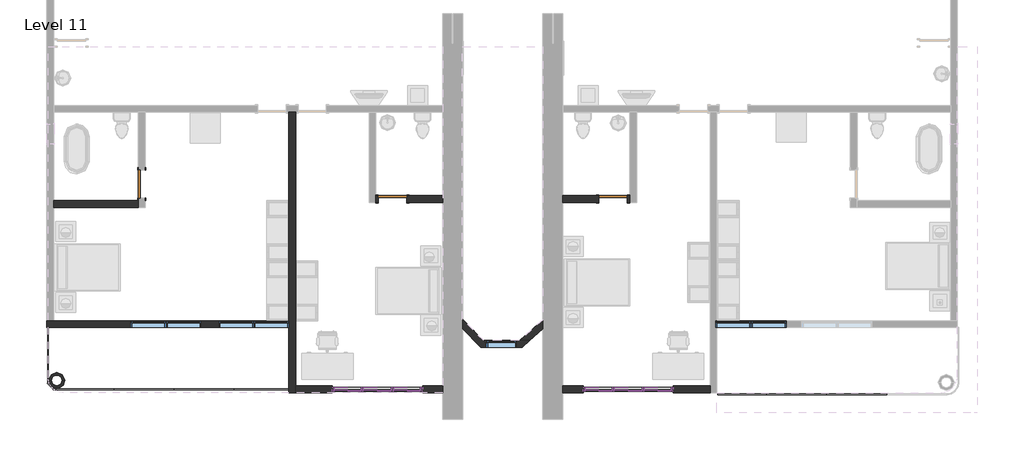
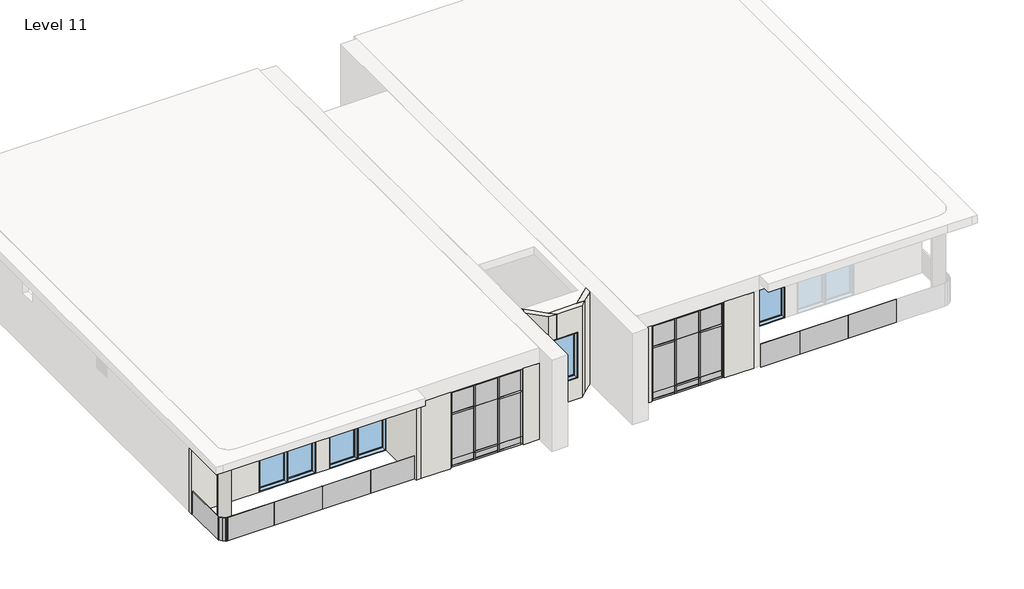
# One storey, part 1 of 3: 42 members, 30 plates, 14 walls, 7 windows, 3 doors.
"""IFC4 building model written with IfcOpenShell, lengths in millimetres."""

from ifc_helpers import new_model, si_unit, point, frame, frame_2d, origin, place, context, project, spatial, polyline, circle_curve, trimmed, segment, composite_curve, outline, extrude, faceted_brep, transform, mapped, element, save
from components import door_2703ae13, door_10fd3a06, member_c17f1be2, member_ad567e07, member_d2e7e466, member_7db1855a, member_75d1e245, member_d60e8053, member_3c3dc66a, member_2fae0574, member_410c6227, member_73c23c35, system_panel_glazed_38d54ecf, system_panel_glazed_fbb6c980, system_panel_glazed_4137532c, system_panel_glazed_6230de04, system_panel_glazed_a79f7f85, system_panel_glazed_9a5ea490, system_panel_glazed_95be5de7, system_panel_glazed_1e00a1c5, system_panel_glazed_ffe51582, system_panel_glazed_8f95e3f6, system_panel_glazed_836907cd, system_panel_glazed_688a65a2, system_panel_glazed_c1a1c740, system_panel_glazed_22bcd51f, window_9a779fa2, window_1a213a25

model = new_model("IFC4")

# Units and contexts
model_context = context("Model", 3, world=origin())
ifc_project = project(units=[si_unit("LENGTHUNIT", "METRE", prefix="MILLI")], contexts=[model_context])

# Site, building, storey
site = spatial("IfcSite", under=ifc_project)
building = spatial("IfcBuilding", under=site)
storey = spatial("IfcBuildingStorey", under=building, Name="Level 11", Elevation=36576.0)

# Doors
placement = place(None, origin())
door_shape = door_2703ae13(model_context)
element("IfcDoor", 1, ObjectType="Door-Single-Panel.0001 : 34\" x 80\"", at=placement, inside=storey, context=model_context, shape_type="MappedRepresentation", body=[
    mapped(door_shape, transform((-15759.6487704, -441.9241442, 36576.0), x_axis=(0.0, -1.0, 0.0), y_axis=(1.0, 0.0, 0.0), z_axis=(0.0, 0.0, 1.0))),
])
element("IfcDoor", 2, ObjectType="Door-Single-Panel.0001 : 34\" x 80\"", at=placement, inside=storey, context=model_context, shape_type="MappedRepresentation", body=[
    mapped(door_shape, transform((-8139.6487704, -899.1241442, 36576.0), x_axis=(-1.0, 0.0, 0.0), y_axis=(0.0, -1.0, 0.0), z_axis=(0.0, 0.0, 1.0))),
])
door_2_shape = door_10fd3a06(model_context)
element("IfcDoor", 3, ObjectType="Door-Single-Panel.0001 : 34\" x 80\"", at=placement, inside=storey, context=model_context, shape_type="MappedRepresentation", body=[
    mapped(door_2_shape, transform((-1434.0487704, -899.1241442, 36576.0), x_axis=(1.0, 0.0, 0.0), y_axis=(0.0, 1.0, 0.0), z_axis=(0.0, 0.0, 1.0))),
])

# Members
member_shape = member_c17f1be2(model_context)
element("IfcMember", 4, ObjectType="Rectangular Mullion : 2.5\" x 5\" rectangular", at=placement, inside=storey, context=model_context, shape_type="MappedRepresentation", body=[
    mapped(member_shape, transform((-9904.9487704, -6690.3241442, 39624.0), x_axis=(0.0, 0.0, 1.0), y_axis=(0.0, 1.0, 0.0), z_axis=(-1.0, 0.0, 0.0))),
])
element("IfcMember", 5, ObjectType="Rectangular Mullion : 2.5\" x 5\" rectangular", at=placement, inside=storey, context=model_context, shape_type="MappedRepresentation", body=[
    mapped(member_shape, transform((-8107.8987704, -6690.3241442, 39624.0), x_axis=(0.0, 0.0, 1.0), y_axis=(0.0, 1.0, 0.0), z_axis=(-1.0, 0.0, 0.0))),
])
element("IfcMember", 6, ObjectType="Rectangular Mullion : 2.5\" x 5\" rectangular", at=placement, inside=storey, context=model_context, shape_type="MappedRepresentation", body=[
    mapped(member_shape, transform((-2284.9487704, -6690.3241442, 39624.0), x_axis=(0.0, 0.0, 1.0), y_axis=(0.0, 1.0, 0.0), z_axis=(-1.0, 0.0, 0.0))),
])
element("IfcMember", 7, ObjectType="Rectangular Mullion : 2.5\" x 5\" rectangular", at=placement, inside=storey, context=model_context, shape_type="MappedRepresentation", body=[
    mapped(member_shape, transform((-487.8987704, -6690.3241442, 39624.0), x_axis=(0.0, 0.0, 1.0), y_axis=(0.0, 1.0, 0.0), z_axis=(-1.0, 0.0, 0.0))),
])
element("IfcMember", 8, ObjectType="Rectangular Mullion : 2.5\" x 5\" rectangular", at=placement, inside=storey, context=model_context, shape_type="MappedRepresentation", body=[
    mapped(member_shape, transform((-7288.7487704, -6690.3241442, 36576.0), x_axis=(0.0, 0.0, -1.0), y_axis=(0.0, 1.0, 0.0), z_axis=(1.0, 0.0, 0.0))),
])
element("IfcMember", 9, ObjectType="Rectangular Mullion : 2.5\" x 5\" rectangular", at=placement, inside=storey, context=model_context, shape_type="MappedRepresentation", body=[
    mapped(member_shape, transform((-9085.7987704, -6690.3241442, 36576.0), x_axis=(0.0, 0.0, -1.0), y_axis=(0.0, 1.0, 0.0), z_axis=(1.0, 0.0, 0.0))),
])
element("IfcMember", 10, ObjectType="Rectangular Mullion : 2.5\" x 5\" rectangular", at=placement, inside=storey, context=model_context, shape_type="MappedRepresentation", body=[
    mapped(member_shape, transform((331.2512296, -6690.3241442, 36576.0), x_axis=(0.0, 0.0, -1.0), y_axis=(0.0, 1.0, 0.0), z_axis=(1.0, 0.0, 0.0))),
])
element("IfcMember", 11, ObjectType="Rectangular Mullion : 2.5\" x 5\" rectangular", at=placement, inside=storey, context=model_context, shape_type="MappedRepresentation", body=[
    mapped(member_shape, transform((-1465.7987704, -6690.3241442, 36576.0), x_axis=(0.0, 0.0, -1.0), y_axis=(0.0, 1.0, 0.0), z_axis=(1.0, 0.0, 0.0))),
])
member_2_shape = member_ad567e07(model_context)
element("IfcMember", 12, ObjectType="Rectangular Mullion : 2.5\" x 5\" rectangular", at=placement, inside=storey, context=model_context, shape_type="MappedRepresentation", body=[
    mapped(member_2_shape, transform((-8107.8987704, -6690.3241442, 38709.6), x_axis=(0.0, 0.0, 1.0), y_axis=(0.0, 1.0, 0.0), z_axis=(-1.0, 0.0, 0.0))),
])
element("IfcMember", 13, ObjectType="Rectangular Mullion : 2.5\" x 5\" rectangular", at=placement, inside=storey, context=model_context, shape_type="MappedRepresentation", body=[
    mapped(member_2_shape, transform((-9904.9487704, -6690.3241442, 38709.6), x_axis=(0.0, 0.0, 1.0), y_axis=(0.0, 1.0, 0.0), z_axis=(-1.0, 0.0, 0.0))),
])
element("IfcMember", 14, ObjectType="Rectangular Mullion : 2.5\" x 5\" rectangular", at=placement, inside=storey, context=model_context, shape_type="MappedRepresentation", body=[
    mapped(member_2_shape, transform((-487.8987704, -6690.3241442, 38709.6), x_axis=(0.0, 0.0, 1.0), y_axis=(0.0, 1.0, 0.0), z_axis=(-1.0, 0.0, 0.0))),
])
element("IfcMember", 15, ObjectType="Rectangular Mullion : 2.5\" x 5\" rectangular", at=placement, inside=storey, context=model_context, shape_type="MappedRepresentation", body=[
    mapped(member_2_shape, transform((-2284.9487704, -6690.3241442, 38709.6), x_axis=(0.0, 0.0, 1.0), y_axis=(0.0, 1.0, 0.0), z_axis=(-1.0, 0.0, 0.0))),
])
member_3_shape = member_d2e7e466(model_context)
element("IfcMember", 16, ObjectType="Rectangular Mullion : 2.5\" x 5\" rectangular", at=placement, inside=storey, context=model_context, shape_type="MappedRepresentation", body=[
    mapped(member_3_shape, transform((-8171.3987704, -6690.3241442, 36576.0), x_axis=(0.0, 0.0, -1.0), y_axis=(0.0, 1.0, 0.0), z_axis=(1.0, 0.0, 0.0))),
])
element("IfcMember", 17, ObjectType="Rectangular Mullion : 2.5\" x 5\" rectangular", at=placement, inside=storey, context=model_context, shape_type="MappedRepresentation", body=[
    mapped(member_3_shape, transform((-551.3987704, -6690.3241442, 36576.0), x_axis=(0.0, 0.0, -1.0), y_axis=(0.0, 1.0, 0.0), z_axis=(1.0, 0.0, 0.0))),
])
member_4_shape = member_7db1855a(model_context)
element("IfcMember", 18, ObjectType="Rectangular Mullion : 2.5\" x 5\" rectangular", at=placement, inside=storey, context=model_context, shape_type="MappedRepresentation", body=[
    mapped(member_4_shape, transform((-9022.2987704, -6690.3241442, 36880.8), x_axis=(0.0, 0.0, 1.0), y_axis=(0.0, 1.0, 0.0), z_axis=(-1.0, 0.0, 0.0))),
])
element("IfcMember", 19, ObjectType="Rectangular Mullion : 2.5\" x 5\" rectangular", at=placement, inside=storey, context=model_context, shape_type="MappedRepresentation", body=[
    mapped(member_4_shape, transform((-1402.2987704, -6690.3241442, 36880.8), x_axis=(0.0, 0.0, 1.0), y_axis=(0.0, 1.0, 0.0), z_axis=(-1.0, 0.0, 0.0))),
])
element("IfcMember", 20, ObjectType="Rectangular Mullion : 2.5\" x 5\" rectangular", at=placement, inside=storey, context=model_context, shape_type="MappedRepresentation", body=[
    mapped(member_3_shape, transform((-9022.2987704, -6690.3241442, 39624.0), x_axis=(0.0, 0.0, 1.0), y_axis=(0.0, 1.0, 0.0), z_axis=(-1.0, 0.0, 0.0))),
])
element("IfcMember", 21, ObjectType="Rectangular Mullion : 2.5\" x 5\" rectangular", at=placement, inside=storey, context=model_context, shape_type="MappedRepresentation", body=[
    mapped(member_3_shape, transform((-1402.2987704, -6690.3241442, 39624.0), x_axis=(0.0, 0.0, 1.0), y_axis=(0.0, 1.0, 0.0), z_axis=(-1.0, 0.0, 0.0))),
])
member_5_shape = member_75d1e245(model_context)
element("IfcMember", 22, ObjectType="Rectangular Mullion : 2.5\" x 5\" rectangular", at=placement, inside=storey, context=model_context, shape_type="MappedRepresentation", body=[
    mapped(member_5_shape, transform((-8139.6487704, -6690.3241442, 36576.0), x_axis=(-1.0, 0.0, 0.0), y_axis=(0.0, 1.0, 0.0), z_axis=(0.0, 0.0, -1.0))),
])
element("IfcMember", 23, ObjectType="Rectangular Mullion : 2.5\" x 5\" rectangular", at=placement, inside=storey, context=model_context, shape_type="MappedRepresentation", body=[
    mapped(member_5_shape, transform((-9054.0487704, -6690.3241442, 36576.0), x_axis=(-1.0, 0.0, 0.0), y_axis=(0.0, 1.0, 0.0), z_axis=(0.0, 0.0, -1.0))),
])
element("IfcMember", 24, ObjectType="Rectangular Mullion : 2.5\" x 5\" rectangular", at=placement, inside=storey, context=model_context, shape_type="MappedRepresentation", body=[
    mapped(member_5_shape, transform((-519.6487704, -6690.3241442, 36576.0), x_axis=(-1.0, 0.0, 0.0), y_axis=(0.0, 1.0, 0.0), z_axis=(0.0, 0.0, -1.0))),
])
element("IfcMember", 25, ObjectType="Rectangular Mullion : 2.5\" x 5\" rectangular", at=placement, inside=storey, context=model_context, shape_type="MappedRepresentation", body=[
    mapped(member_5_shape, transform((-1434.0487704, -6690.3241442, 36576.0), x_axis=(-1.0, 0.0, 0.0), y_axis=(0.0, 1.0, 0.0), z_axis=(0.0, 0.0, -1.0))),
])
member_6_shape = member_d60e8053(model_context)
element("IfcMember", 26, ObjectType="Rectangular Mullion : 2.5\" x 5\" rectangular", at=placement, inside=storey, context=model_context, shape_type="MappedRepresentation", body=[
    mapped(member_6_shape, transform((-8139.6487704, -6690.3241442, 36880.8), x_axis=(-1.0, 0.0, 0.0), y_axis=(0.0, 1.0, 0.0), z_axis=(0.0, 0.0, -1.0))),
])
element("IfcMember", 27, ObjectType="Rectangular Mullion : 2.5\" x 5\" rectangular", at=placement, inside=storey, context=model_context, shape_type="MappedRepresentation", body=[
    mapped(member_6_shape, transform((-9054.0487704, -6690.3241442, 36880.8), x_axis=(-1.0, 0.0, 0.0), y_axis=(0.0, 1.0, 0.0), z_axis=(0.0, 0.0, -1.0))),
])
element("IfcMember", 28, ObjectType="Rectangular Mullion : 2.5\" x 5\" rectangular", at=placement, inside=storey, context=model_context, shape_type="MappedRepresentation", body=[
    mapped(member_6_shape, transform((-519.6487704, -6690.3241442, 36880.8), x_axis=(-1.0, 0.0, 0.0), y_axis=(0.0, 1.0, 0.0), z_axis=(0.0, 0.0, -1.0))),
])
element("IfcMember", 29, ObjectType="Rectangular Mullion : 2.5\" x 5\" rectangular", at=placement, inside=storey, context=model_context, shape_type="MappedRepresentation", body=[
    mapped(member_6_shape, transform((-1434.0487704, -6690.3241442, 36880.8), x_axis=(-1.0, 0.0, 0.0), y_axis=(0.0, 1.0, 0.0), z_axis=(0.0, 0.0, -1.0))),
])
member_7_shape = member_3c3dc66a(model_context)
element("IfcMember", 30, ObjectType="Rectangular Mullion : 2.5\" x 5\" rectangular", at=placement, inside=storey, context=model_context, shape_type="MappedRepresentation", body=[
    mapped(member_7_shape, transform((-9968.4487704, -6690.3241442, 36576.0), x_axis=(-1.0, 0.0, 0.0), y_axis=(0.0, 1.0, 0.0), z_axis=(0.0, 0.0, -1.0))),
])
element("IfcMember", 31, ObjectType="Rectangular Mullion : 2.5\" x 5\" rectangular", at=placement, inside=storey, context=model_context, shape_type="MappedRepresentation", body=[
    mapped(member_7_shape, transform((-2348.4487704, -6690.3241442, 36576.0), x_axis=(-1.0, 0.0, 0.0), y_axis=(0.0, 1.0, 0.0), z_axis=(0.0, 0.0, -1.0))),
])
member_8_shape = member_2fae0574(model_context)
element("IfcMember", 32, ObjectType="Rectangular Mullion : 2.5\" x 5\" rectangular", at=placement, inside=storey, context=model_context, shape_type="MappedRepresentation", body=[
    mapped(member_8_shape, transform((-9968.4487704, -6690.3241442, 36880.8), x_axis=(-1.0, 0.0, 0.0), y_axis=(0.0, 1.0, 0.0), z_axis=(0.0, 0.0, -1.0))),
])
element("IfcMember", 33, ObjectType="Rectangular Mullion : 2.5\" x 5\" rectangular", at=placement, inside=storey, context=model_context, shape_type="MappedRepresentation", body=[
    mapped(member_8_shape, transform((-2348.4487704, -6690.3241442, 36880.8), x_axis=(-1.0, 0.0, 0.0), y_axis=(0.0, 1.0, 0.0), z_axis=(0.0, 0.0, -1.0))),
])
element("IfcMember", 34, ObjectType="Rectangular Mullion : 2.5\" x 5\" rectangular", at=placement, inside=storey, context=model_context, shape_type="MappedRepresentation", body=[
    mapped(member_8_shape, transform((-7225.2487704, -6690.3241442, 38709.6), x_axis=(1.0, 0.0, 0.0), y_axis=(0.0, 1.0, 0.0), z_axis=(0.0, 0.0, 1.0))),
])
element("IfcMember", 35, ObjectType="Rectangular Mullion : 2.5\" x 5\" rectangular", at=placement, inside=storey, context=model_context, shape_type="MappedRepresentation", body=[
    mapped(member_8_shape, transform((394.7512296, -6690.3241442, 38709.6), x_axis=(1.0, 0.0, 0.0), y_axis=(0.0, 1.0, 0.0), z_axis=(0.0, 0.0, 1.0))),
])
element("IfcMember", 36, ObjectType="Rectangular Mullion : 2.5\" x 5\" rectangular", at=placement, inside=storey, context=model_context, shape_type="MappedRepresentation", body=[
    mapped(member_7_shape, transform((-7225.2487704, -6690.3241442, 36880.8), x_axis=(1.0, 0.0, 0.0), y_axis=(0.0, 1.0, 0.0), z_axis=(0.0, 0.0, 1.0))),
])
element("IfcMember", 37, ObjectType="Rectangular Mullion : 2.5\" x 5\" rectangular", at=placement, inside=storey, context=model_context, shape_type="MappedRepresentation", body=[
    mapped(member_7_shape, transform((394.7512296, -6690.3241442, 36880.8), x_axis=(1.0, 0.0, 0.0), y_axis=(0.0, 1.0, 0.0), z_axis=(0.0, 0.0, 1.0))),
])
member_9_shape = member_410c6227(model_context)
element("IfcMember", 38, ObjectType="Rectangular Mullion : 2.5\" x 5\" rectangular", at=placement, inside=storey, context=model_context, shape_type="MappedRepresentation", body=[
    mapped(member_9_shape, transform((-8139.6487704, -6690.3241442, 38709.6), x_axis=(-1.0, 0.0, 0.0), y_axis=(0.0, 1.0, 0.0), z_axis=(0.0, 0.0, -1.0))),
])
element("IfcMember", 39, ObjectType="Rectangular Mullion : 2.5\" x 5\" rectangular", at=placement, inside=storey, context=model_context, shape_type="MappedRepresentation", body=[
    mapped(member_9_shape, transform((-9054.0487704, -6690.3241442, 38709.6), x_axis=(-1.0, 0.0, 0.0), y_axis=(0.0, 1.0, 0.0), z_axis=(0.0, 0.0, -1.0))),
])
element("IfcMember", 40, ObjectType="Rectangular Mullion : 2.5\" x 5\" rectangular", at=placement, inside=storey, context=model_context, shape_type="MappedRepresentation", body=[
    mapped(member_9_shape, transform((-519.6487704, -6690.3241442, 38709.6), x_axis=(-1.0, 0.0, 0.0), y_axis=(0.0, 1.0, 0.0), z_axis=(0.0, 0.0, -1.0))),
])
element("IfcMember", 41, ObjectType="Rectangular Mullion : 2.5\" x 5\" rectangular", at=placement, inside=storey, context=model_context, shape_type="MappedRepresentation", body=[
    mapped(member_9_shape, transform((-1434.0487704, -6690.3241442, 38709.6), x_axis=(-1.0, 0.0, 0.0), y_axis=(0.0, 1.0, 0.0), z_axis=(0.0, 0.0, -1.0))),
])
member_10_shape = member_73c23c35(model_context)
element("IfcMember", 42, ObjectType="Rectangular Mullion : 2.5\" x 5\" rectangular", at=placement, inside=storey, context=model_context, shape_type="MappedRepresentation", body=[
    mapped(member_10_shape, transform((-7225.2487704, -6690.3241442, 39624.0), x_axis=(1.0, 0.0, 0.0), y_axis=(0.0, 1.0, 0.0), z_axis=(0.0, 0.0, 1.0))),
])
element("IfcMember", 43, ObjectType="Rectangular Mullion : 2.5\" x 5\" rectangular", at=placement, inside=storey, context=model_context, shape_type="MappedRepresentation", body=[
    mapped(member_10_shape, transform((394.7512296, -6690.3241442, 39624.0), x_axis=(1.0, 0.0, 0.0), y_axis=(0.0, 1.0, 0.0), z_axis=(0.0, 0.0, 1.0))),
])
element("IfcMember", 44, ObjectType="Rectangular Mullion : 2.5\" x 5\" rectangular", at=placement, inside=storey, context=model_context, shape_type="MappedRepresentation", body=[
    mapped(member_10_shape, transform((-9968.4487704, -6690.3241442, 38709.6), x_axis=(-1.0, 0.0, 0.0), y_axis=(0.0, 1.0, 0.0), z_axis=(0.0, 0.0, -1.0))),
])
element("IfcMember", 45, ObjectType="Rectangular Mullion : 2.5\" x 5\" rectangular", at=placement, inside=storey, context=model_context, shape_type="MappedRepresentation", body=[
    mapped(member_10_shape, transform((-2348.4487704, -6690.3241442, 38709.6), x_axis=(-1.0, 0.0, 0.0), y_axis=(0.0, 1.0, 0.0), z_axis=(0.0, 0.0, -1.0))),
])

# Plates
system_panel_glazed_shape = system_panel_glazed_38d54ecf(model_context)
element("IfcPlate", 46, ObjectType="System Panel : Glazed", at=placement, inside=storey, context=model_context, shape_type="MappedRepresentation", body=[
    mapped(system_panel_glazed_shape, transform((-8596.8487704, -6690.3241442, 36912.55), x_axis=(-1.0, 0.0, 0.0), y_axis=(0.0, -1.0, 0.0), z_axis=(0.0, 0.0, 1.0))),
])
element("IfcPlate", 47, ObjectType="System Panel : Glazed", at=placement, inside=storey, context=model_context, shape_type="MappedRepresentation", body=[
    mapped(system_panel_glazed_shape, transform((-976.8487704, -6690.3241442, 36912.55), x_axis=(-1.0, 0.0, 0.0), y_axis=(0.0, -1.0, 0.0), z_axis=(0.0, 0.0, 1.0))),
])
system_panel_glazed_2_shape = system_panel_glazed_fbb6c980(model_context)
element("IfcPlate", 48, ObjectType="System Panel : Glazed", at=placement, inside=storey, context=model_context, shape_type="MappedRepresentation", body=[
    mapped(system_panel_glazed_2_shape, transform((-8596.8487704, -6690.3241442, 36639.5), x_axis=(-1.0, 0.0, 0.0), y_axis=(0.0, -1.0, 0.0), z_axis=(0.0, 0.0, 1.0))),
])
element("IfcPlate", 49, ObjectType="System Panel : Glazed", at=placement, inside=storey, context=model_context, shape_type="MappedRepresentation", body=[
    mapped(system_panel_glazed_2_shape, transform((-976.8487704, -6690.3241442, 36639.5), x_axis=(-1.0, 0.0, 0.0), y_axis=(0.0, -1.0, 0.0), z_axis=(0.0, 0.0, 1.0))),
])
system_panel_glazed_3_shape = system_panel_glazed_4137532c(model_context)
element("IfcPlate", 50, ObjectType="System Panel : Glazed", at=placement, inside=storey, context=model_context, shape_type="MappedRepresentation", body=[
    mapped(system_panel_glazed_3_shape, transform((-7698.3237704, -6690.3241442, 36639.5), x_axis=(-1.0, 0.0, 0.0), y_axis=(0.0, -1.0, 0.0), z_axis=(0.0, 0.0, 1.0))),
])
element("IfcPlate", 51, ObjectType="System Panel : Glazed", at=placement, inside=storey, context=model_context, shape_type="MappedRepresentation", body=[
    mapped(system_panel_glazed_3_shape, transform((-9495.3737704, -6690.3241442, 36639.5), x_axis=(-1.0, 0.0, 0.0), y_axis=(0.0, -1.0, 0.0), z_axis=(0.0, 0.0, 1.0))),
])
element("IfcPlate", 52, ObjectType="System Panel : Glazed", at=placement, inside=storey, context=model_context, shape_type="MappedRepresentation", body=[
    mapped(system_panel_glazed_3_shape, transform((-78.3237704, -6690.3241442, 36639.5), x_axis=(-1.0, 0.0, 0.0), y_axis=(0.0, -1.0, 0.0), z_axis=(0.0, 0.0, 1.0))),
])
element("IfcPlate", 53, ObjectType="System Panel : Glazed", at=placement, inside=storey, context=model_context, shape_type="MappedRepresentation", body=[
    mapped(system_panel_glazed_3_shape, transform((-1875.3737704, -6690.3241442, 36639.5), x_axis=(-1.0, 0.0, 0.0), y_axis=(0.0, -1.0, 0.0), z_axis=(0.0, 0.0, 1.0))),
])
system_panel_glazed_4_shape = system_panel_glazed_6230de04(model_context)
element("IfcPlate", 54, ObjectType="System Panel : Glazed", at=placement, inside=storey, context=model_context, shape_type="MappedRepresentation", body=[
    mapped(system_panel_glazed_4_shape, transform((-7698.3237704, -6690.3241442, 36880.8), x_axis=(-1.0, 0.0, 0.0), y_axis=(0.0, -1.0, 0.0), z_axis=(0.0, 0.0, 1.0))),
])
element("IfcPlate", 55, ObjectType="System Panel : Glazed", at=placement, inside=storey, context=model_context, shape_type="MappedRepresentation", body=[
    mapped(system_panel_glazed_4_shape, transform((-9495.3737704, -6690.3241442, 36880.8), x_axis=(-1.0, 0.0, 0.0), y_axis=(0.0, -1.0, 0.0), z_axis=(0.0, 0.0, 1.0))),
])
element("IfcPlate", 56, ObjectType="System Panel : Glazed", at=placement, inside=storey, context=model_context, shape_type="MappedRepresentation", body=[
    mapped(system_panel_glazed_4_shape, transform((-78.3237704, -6690.3241442, 36880.8), x_axis=(-1.0, 0.0, 0.0), y_axis=(0.0, -1.0, 0.0), z_axis=(0.0, 0.0, 1.0))),
])
element("IfcPlate", 57, ObjectType="System Panel : Glazed", at=placement, inside=storey, context=model_context, shape_type="MappedRepresentation", body=[
    mapped(system_panel_glazed_4_shape, transform((-1875.3737704, -6690.3241442, 36880.8), x_axis=(-1.0, 0.0, 0.0), y_axis=(0.0, -1.0, 0.0), z_axis=(0.0, 0.0, 1.0))),
])
system_panel_glazed_5_shape = system_panel_glazed_a79f7f85(model_context)
element("IfcPlate", 58, ObjectType="System Panel : Glazed", at=placement, inside=storey, context=model_context, shape_type="MappedRepresentation", body=[
    mapped(system_panel_glazed_5_shape, transform((-7698.3237704, -6690.3241442, 38741.35), x_axis=(-1.0, 0.0, 0.0), y_axis=(0.0, -1.0, 0.0), z_axis=(0.0, 0.0, 1.0))),
])
element("IfcPlate", 59, ObjectType="System Panel : Glazed", at=placement, inside=storey, context=model_context, shape_type="MappedRepresentation", body=[
    mapped(system_panel_glazed_5_shape, transform((-9495.3737704, -6690.3241442, 38741.35), x_axis=(-1.0, 0.0, 0.0), y_axis=(0.0, -1.0, 0.0), z_axis=(0.0, 0.0, 1.0))),
])
element("IfcPlate", 60, ObjectType="System Panel : Glazed", at=placement, inside=storey, context=model_context, shape_type="MappedRepresentation", body=[
    mapped(system_panel_glazed_5_shape, transform((-78.3237704, -6690.3241442, 38741.35), x_axis=(-1.0, 0.0, 0.0), y_axis=(0.0, -1.0, 0.0), z_axis=(0.0, 0.0, 1.0))),
])
element("IfcPlate", 61, ObjectType="System Panel : Glazed", at=placement, inside=storey, context=model_context, shape_type="MappedRepresentation", body=[
    mapped(system_panel_glazed_5_shape, transform((-1875.3737704, -6690.3241442, 38741.35), x_axis=(-1.0, 0.0, 0.0), y_axis=(0.0, -1.0, 0.0), z_axis=(0.0, 0.0, 1.0))),
])
system_panel_glazed_6_shape = system_panel_glazed_9a5ea490(model_context)
element("IfcPlate", 62, ObjectType="System Panel : Glazed", at=placement, inside=storey, context=model_context, shape_type="MappedRepresentation", body=[
    mapped(system_panel_glazed_6_shape, transform((-8596.8487704, -6690.3241442, 38709.6), x_axis=(-1.0, 0.0, 0.0), y_axis=(0.0, -1.0, 0.0), z_axis=(0.0, 0.0, 1.0))),
])
element("IfcPlate", 63, ObjectType="System Panel : Glazed", at=placement, inside=storey, context=model_context, shape_type="MappedRepresentation", body=[
    mapped(system_panel_glazed_6_shape, transform((-976.8487704, -6690.3241442, 38709.6), x_axis=(-1.0, 0.0, 0.0), y_axis=(0.0, -1.0, 0.0), z_axis=(0.0, 0.0, 1.0))),
])
system_panel_glazed_7_shape = system_panel_glazed_95be5de7(model_context)
element("IfcPlate", 64, ObjectType="System Panel : Glazed", at=placement, inside=storey, context=model_context, shape_type="MappedRepresentation", body=[
    mapped(system_panel_glazed_7_shape, transform((-15700.8805745, -6723.6923401, 36576.0), x_axis=(1.0, 0.0, 0.0), y_axis=(0.0, 1.0, 0.0), z_axis=(0.0, 0.0, 1.0))),
])
element("IfcPlate", 65, ObjectType="System Panel : Glazed", at=placement, inside=storey, context=model_context, shape_type="MappedRepresentation", body=[
    mapped(system_panel_glazed_7_shape, transform((-13872.0805745, -6723.6923401, 36576.0), x_axis=(1.0, 0.0, 0.0), y_axis=(0.0, 1.0, 0.0), z_axis=(0.0, 0.0, 1.0))),
])
element("IfcPlate", 66, ObjectType="System Panel : Glazed", at=placement, inside=storey, context=model_context, shape_type="MappedRepresentation", body=[
    mapped(system_panel_glazed_7_shape, transform((5964.2620092, -6810.4133646, 36576.0), x_axis=(-1.0, 0.0, 0.0), y_axis=(0.0, -1.0, 0.0), z_axis=(0.0, 0.0, 1.0))),
])
element("IfcPlate", 67, ObjectType="System Panel : Glazed", at=placement, inside=storey, context=model_context, shape_type="MappedRepresentation", body=[
    mapped(system_panel_glazed_7_shape, transform((4135.4620092, -6810.4133646, 36576.0), x_axis=(-1.0, 0.0, 0.0), y_axis=(0.0, -1.0, 0.0), z_axis=(0.0, 0.0, 1.0))),
])
system_panel_glazed_8_shape = system_panel_glazed_1e00a1c5(model_context)
element("IfcPlate", 68, ObjectType="System Panel : Glazed", at=placement, inside=storey, context=model_context, shape_type="MappedRepresentation", body=[
    mapped(system_panel_glazed_8_shape, transform((2484.4620092, -6810.4133646, 36576.0), x_axis=(-1.0, 0.0, 0.0), y_axis=(0.0, -1.0, 0.0), z_axis=(0.0, 0.0, 1.0))),
])
system_panel_glazed_9_shape = system_panel_glazed_ffe51582(model_context)
element("IfcPlate", 69, ObjectType="System Panel : Glazed", at=placement, inside=storey, context=model_context, shape_type="MappedRepresentation", body=[
    mapped(system_panel_glazed_9_shape, transform((-18445.6213429, -6722.1515718, 36576.0), x_axis=(0.7071067811865462, -0.7071067811865488, 0.0), y_axis=(0.7071067811865488, 0.7071067811865462, 0.0), z_axis=(0.0, 0.0, 1.0))),
])
system_panel_glazed_10_shape = system_panel_glazed_8f95e3f6(model_context)
element("IfcPlate", 70, ObjectType="System Panel : Glazed", at=placement, inside=storey, context=model_context, shape_type="MappedRepresentation", body=[
    mapped(system_panel_glazed_10_shape, transform((-18642.5487704, -5667.9741442, 36576.0), x_axis=(0.0, -1.0, 0.0), y_axis=(1.0, 0.0, 0.0), z_axis=(0.0, 0.0, 1.0))),
])
system_panel_glazed_11_shape = system_panel_glazed_836907cd(model_context)
element("IfcPlate", 71, ObjectType="System Panel : Glazed", at=placement, inside=storey, context=model_context, shape_type="MappedRepresentation", body=[
    mapped(system_panel_glazed_11_shape, transform((-18412.3305745, -6723.6923401, 36576.0), x_axis=(1.0, 0.0, 0.0), y_axis=(0.0, 1.0, 0.0), z_axis=(0.0, 0.0, 1.0))),
])
system_panel_glazed_12_shape = system_panel_glazed_688a65a2(model_context)
element("IfcPlate", 72, ObjectType="System Panel : Glazed", at=placement, inside=storey, context=model_context, shape_type="MappedRepresentation", body=[
    mapped(system_panel_glazed_12_shape, transform((-12123.4646725, -6723.6923401, 36576.0), x_axis=(1.0, 0.0, 0.0), y_axis=(0.0, 1.0, 0.0), z_axis=(0.0, 0.0, 1.0))),
])
system_panel_glazed_13_shape = system_panel_glazed_c1a1c740(model_context)
element("IfcPlate", 73, ObjectType="System Panel : Glazed", at=placement, inside=storey, context=model_context, shape_type="MappedRepresentation", body=[
    mapped(system_panel_glazed_13_shape, transform((-17497.9305745, -6723.6923401, 36576.0), x_axis=(1.0, 0.0, 0.0), y_axis=(0.0, 1.0, 0.0), z_axis=(0.0, 0.0, 1.0))),
])
system_panel_glazed_14_shape = system_panel_glazed_22bcd51f(model_context)
element("IfcPlate", 74, ObjectType="System Panel : Glazed", at=placement, inside=storey, context=model_context, shape_type="MappedRepresentation", body=[
    mapped(system_panel_glazed_14_shape, transform((-18593.7021056, -6574.070809, 36576.0), x_axis=(0.7071067811865462, -0.7071067811865488, 0.0), y_axis=(0.7071067811865488, 0.7071067811865462, 0.0), z_axis=(0.0, 0.0, 1.0))),
])
element("IfcPlate", 75, ObjectType="System Panel : Glazed", at=placement, inside=storey, context=model_context, shape_type="MappedRepresentation", body=[
    mapped(system_panel_glazed_14_shape, transform((-18496.0087761, -6671.7641386, 36576.0), x_axis=(0.7071067811865462, -0.7071067811865488, 0.0), y_axis=(0.7071067811865488, 0.7071067811865462, 0.0), z_axis=(0.0, 0.0, 1.0))),
])

# Walls
element("IfcWall", 76, ObjectType="Generic - 3\" green 2", at=placement, inside=storey, context=model_context, shape_type="SweptSolid", body=[
    extrude(outline(composite_curve([segment(polyline([(-18512.3737704, -6418.8616442), (-18588.5737704, -6418.8616442)]), True, "CONTINUOUS"), segment(trimmed(circle_curve(frame_2d((-18347.2737704, -6418.8616442)), 241.3), [point((-18588.5737704, -6418.8616442))], [point((-18105.9737704, -6418.8616442))], False, "CARTESIAN"), True, "CONTINUOUS"), segment(polyline([(-18105.9737704, -6418.8616442), (-18182.1737704, -6418.8616442)]), True, "CONTINUOUS"), segment(trimmed(circle_curve(frame_2d((-18347.2737704, -6418.8616442)), 165.1), [point((-18182.1737704, -6418.8616442))], [point((-18512.3737704, -6418.8616442))], True, "CARTESIAN"), True, "CONTINUOUS")], self_intersect=False)), frame((0.0, 0.0, 36576.0), z_axis=(0.0, 0.0, 1.0), x_axis=(1.0, 0.0, 0.0)), (0.0, 0.0, 1.0), 3048.0),
])
element("IfcWall", 77, ObjectType="Generic - 3\" green 2", at=placement, inside=storey, context=model_context, shape_type="SweptSolid", body=[
    extrude(outline(composite_curve([segment(polyline([(-18182.1737704, -6418.8616442), (-18105.9737704, -6418.8616442)]), True, "CONTINUOUS"), segment(trimmed(circle_curve(frame_2d((-18347.2737704, -6418.8616442)), 241.3), [point((-18105.9737704, -6418.8616442))], [point((-18588.5737704, -6418.8616442))], False, "CARTESIAN"), True, "CONTINUOUS"), segment(polyline([(-18588.5737704, -6418.8616442), (-18512.3737704, -6418.8616442)]), True, "CONTINUOUS"), segment(trimmed(circle_curve(frame_2d((-18347.2737704, -6418.8616442)), 165.1), [point((-18512.3737704, -6418.8616442))], [point((-18182.1737704, -6418.8616442))], True, "CARTESIAN"), True, "CONTINUOUS")], self_intersect=False)), frame((0.0, 0.0, 36576.0), z_axis=(0.0, 0.0, 1.0), x_axis=(1.0, 0.0, 0.0)), (0.0, 0.0, 1.0), 3048.0),
])
element("IfcWall", 78, ObjectType="Generic - 8\" cream", at=placement, inside=storey, context=model_context, shape_type="Brep", body=[
    faceted_brep([(-11289.2487704, 1742.4758558, 36576.0), (-11289.2487704, -6791.9241442, 36576.0), (-11289.2487704, -6791.9241442, 39624.0), (-11289.2487704, -4810.7241442, 39624.0), (-11289.2487704, -4607.5241442, 39624.0), (-11289.2487704, 1742.4758558, 39624.0), (-11086.0487704, 1742.4758558, 36576.0), (-11086.0487704, 1742.4758558, 39624.0), (-11086.0487704, -6588.7241442, 39624.0), (-11086.0487704, -6791.9241442, 39624.0), (-11086.0487704, -6791.9241442, 36576.0), (-11086.0487704, -6588.7241442, 36576.0)], [[[0, 1, 2, 3, 4, 5]], [[6, 7, 8, 9, 10, 11]], [[1, 0, 6, 11, 10]], [[5, 4, 3, 2, 9, 8, 7]], [[0, 5, 7, 6]], [[2, 1, 10, 9]]]),
])
element("IfcWall", 79, ObjectType="Generic - 8\" cream", at=placement, inside=storey, context=model_context, shape_type="SweptSolid", body=[
    extrude(outline(polyline([(-18439.3487704, -949.9241442), (-15861.2487704, -949.9241442), (-15861.2487704, -1153.1241442), (-18439.3487704, -1153.1241442), (-18439.3487704, -949.9241442)])), frame((0.0, 0.0, 36576.0), z_axis=(0.0, 0.0, 1.0), x_axis=(1.0, 0.0, 0.0)), (0.0, 0.0, 1.0), 3048.0),
])
element("IfcWall", 80, ObjectType="Generic - 8\" cream", at=placement, inside=storey, context=model_context, shape_type="SweptSolid", body=[
    extrude(outline(polyline([(39624.0, -6615.6487704), (39624.0, -8647.6487704), (36576.0, -8647.6487704), (36576.0, -8571.4487704), (38608.0, -8571.4487704), (38608.0, -7707.8487704), (36576.0, -7707.8487704), (36576.0, -6615.6487704), (39624.0, -6615.6487704)])), frame((0.0, -1000.7241442, 0.0), z_axis=(0.0, 1.0, 0.0), x_axis=(0.0, 0.0, 1.0)), (0.0, 0.0, 1.0), 203.2),
])
element("IfcWall", 81, ObjectType="Generic - 8\" cream", at=placement, inside=storey, context=model_context, shape_type="Brep", body=[
    faceted_brep([(-18642.5487704, -4607.5241442, 39624.0), (-18439.3487704, -4607.5241442, 39624.0), (-11289.2487704, -4607.5241442, 39624.0), (-11289.2487704, -4607.5241442, 39319.2), (-13422.8487704, -4607.5241442, 39319.2), (-13422.8487704, -4607.5241442, 36576.0), (-13956.2487704, -4607.5241442, 36576.0), (-13956.2487704, -4607.5241442, 39319.2), (-16089.8487704, -4607.5241442, 39319.2), (-16089.8487704, -4607.5241442, 36576.0), (-18439.3487704, -4607.5241442, 36576.0), (-18642.5487704, -4607.5241442, 36576.0), (-11289.2487704, -4810.7241442, 39624.0), (-18642.5487704, -4810.7241442, 39624.0), (-18642.5487704, -4810.7241442, 36576.0), (-16089.8487704, -4810.7241442, 36576.0), (-16089.8487704, -4810.7241442, 39319.2), (-13956.2487704, -4810.7241442, 39319.2), (-13956.2487704, -4810.7241442, 36576.0), (-13422.8487704, -4810.7241442, 36576.0), (-13422.8487704, -4810.7241442, 39319.2), (-11289.2487704, -4810.7241442, 39319.2)], [[[0, 1, 2, 3, 4, 5, 6, 7, 8, 9, 10, 11]], [[12, 13, 14, 15, 16, 17, 18, 19, 20, 21]], [[14, 11, 10, 9, 15]], [[5, 19, 18, 6]], [[2, 1, 0, 13, 12]], [[2, 12, 21, 3]], [[0, 11, 14, 13]], [[3, 21, 20, 4]], [[4, 20, 19, 5]], [[17, 7, 6, 18]], [[7, 17, 16, 8]], [[8, 16, 15, 9]]]),
])
element("IfcWall", 82, ObjectType="Generic - 8\" cream", at=placement, inside=storey, context=model_context, shape_type="SweptSolid", body=[
    extrude(outline(polyline([(39624.0, -926.0487704), (39624.0, -2958.0487704), (36576.0, -2958.0487704), (36576.0, -1865.8487704), (38608.0, -1865.8487704), (38608.0, -1002.2487704), (36576.0, -1002.2487704), (36576.0, -926.0487704), (39624.0, -926.0487704)])), frame((0.0, -1000.7241442, 0.0), z_axis=(0.0, 1.0, 0.0), x_axis=(0.0, 0.0, 1.0)), (0.0, 0.0, 1.0), 203.2),
])
element("IfcWall", 83, ObjectType="Generic - 8\" cream", at=placement, inside=storey, context=model_context, shape_type="SweptSolid", body=[
    extrude(outline(polyline([(394.7512296, -6588.7241442), (1512.3512296, -6588.7241442), (1512.3512296, -6791.9241442), (394.7512296, -6791.9241442), (394.7512296, -6588.7241442)])), frame((0.0, 0.0, 36576.0), z_axis=(0.0, 0.0, 1.0), x_axis=(1.0, 0.0, 0.0)), (0.0, 0.0, 1.0), 3048.0),
])
element("IfcWall", 84, ObjectType="Generic - 8\" cream", at=placement, inside=storey, context=model_context, shape_type="SweptSolid", body=[
    extrude(outline(polyline([(-2348.4487704, -6791.9241442), (-2958.0487704, -6791.9241442), (-2958.0487704, -6588.7241442), (-2348.4487704, -6588.7241442), (-2348.4487704, -6791.9241442)])), frame((0.0, 0.0, 36576.0), z_axis=(0.0, 0.0, 1.0), x_axis=(1.0, 0.0, 0.0)), (0.0, 0.0, 1.0), 3048.0),
])
element("IfcWall", 85, ObjectType="Generic - 8\" cream", at=placement, inside=storey, context=model_context, shape_type="SweptSolid", body=[
    extrude(outline(polyline([(-9968.4487704, -6791.9241442), (-11086.0487704, -6791.9241442), (-11086.0487704, -6588.7241442), (-9968.4487704, -6588.7241442), (-9968.4487704, -6791.9241442)])), frame((0.0, 0.0, 36576.0), z_axis=(0.0, 0.0, 1.0), x_axis=(1.0, 0.0, 0.0)), (0.0, 0.0, 1.0), 3048.0),
])
element("IfcWall", 86, ObjectType="Generic - 8\" cream", at=placement, inside=storey, context=model_context, shape_type="SweptSolid", body=[
    extrude(outline(polyline([(-7225.2487704, -6588.7241442), (-6615.6487704, -6588.7241442), (-6615.6487704, -6791.9241442), (-7225.2487704, -6791.9241442), (-7225.2487704, -6588.7241442)])), frame((0.0, 0.0, 36576.0), z_axis=(0.0, 0.0, 1.0), x_axis=(1.0, 0.0, 0.0)), (0.0, 0.0, 1.0), 3048.0),
])
element("IfcWall", 87, ObjectType="Generic - 8\" green", at=placement, inside=storey, context=model_context, shape_type="Brep", body=[
    faceted_brep([(-6006.0487704, -4852.8082422, 36576.0), (-5452.3544276, -5406.502585, 36576.0), (-5452.3544276, -5406.502585, 40233.6), (-6006.0487704, -4852.8082422, 40233.6), (-5164.9862318, -5406.502585, 36576.0), (-5368.1862318, -5203.302585, 36576.0), (-6006.0487704, -4565.4400463, 36576.0), (-6006.0487704, -4565.4400463, 40233.6), (-5368.1862318, -5203.302585, 40233.6), (-5164.9862318, -5406.502585, 40233.6), (-5164.9862318, -5406.502585, 39243.0), (-5283.1401401, -5288.3486766, 39243.0), (-5283.1401401, -5288.3486766, 37414.2), (-5164.9862318, -5406.502585, 37414.2), (-5283.1401401, -5406.502585, 37414.2), (-5283.1401401, -5406.502585, 39243.0)], [[[0, 1, 2, 3]], [[4, 5, 6, 7, 8, 9, 10, 11, 12, 13]], [[1, 0, 6, 5, 4]], [[3, 2, 9, 8, 7]], [[0, 3, 7, 6]], [[2, 1, 4, 13, 14, 15, 10, 9]], [[12, 14, 13]], [[14, 12, 11, 15]], [[15, 11, 10]]]),
])
element("IfcWall", 88, ObjectType="Generic - 8\" green", at=placement, inside=storey, context=model_context, shape_type="Brep", body=[
    faceted_brep([(-5164.9862318, -5406.502585, 36576.0), (-4196.9843712, -5406.502585, 36576.0), (-4196.9843712, -5406.502585, 40233.6), (-5164.9862318, -5406.502585, 40233.6), (-5164.9862318, -5406.502585, 39243.0), (-4368.7401401, -5406.502585, 39243.0), (-4368.7401401, -5406.502585, 37414.2), (-5164.9862318, -5406.502585, 37414.2), (-3969.1320774, -5203.302585, 36576.0), (-4274.4301413, -5203.302585, 36576.0), (-5368.1862318, -5203.302585, 36576.0), (-5368.1862318, -5203.302585, 40233.6), (-4274.4301413, -5203.302585, 40233.6), (-3969.1320774, -5203.302585, 40233.6), (-4368.7401401, -5203.302585, 37414.2), (-4368.7401401, -5203.302585, 39243.0), (-5283.1401401, -5203.302585, 39243.0), (-5283.1401401, -5203.302585, 37414.2), (-5283.1401401, -5288.3486766, 37414.2), (-5283.1401401, -5288.3486766, 39243.0)], [[[0, 1, 2, 3, 4, 5, 6, 7]], [[8, 9, 10, 11, 12, 13], [14, 15, 16, 17]], [[1, 0, 10, 9, 8]], [[3, 2, 13, 12, 11]], [[3, 11, 10, 0, 7, 18, 19, 4]], [[2, 1, 8, 13]], [[5, 15, 14, 6]], [[6, 14, 17, 18, 7]], [[18, 17, 16, 19]], [[15, 5, 4, 19, 16]]]),
])
element("IfcWall", 89, ObjectType="Generic - 8\" green", at=placement, inside=storey, context=model_context, shape_type="SweptSolid", body=[
    extrude(outline(polyline([(-3567.6487704, -4845.2574382), (-3969.1320774, -5203.302585), (-4274.4301413, -5203.302585), (-3567.6487704, -4572.9908503), (-3567.6487704, -4845.2574382)])), frame((0.0, 0.0, 36576.0), z_axis=(0.0, 0.0, 1.0), x_axis=(1.0, 0.0, 0.0)), (0.0, 0.0, 1.0), 3657.6),
])

# Windows
window_shape = window_9a779fa2(model_context)
element("IfcWindow", 90, ObjectType="Fixed : 36\" x 72\"", at=placement, inside=storey, context=model_context, shape_type="MappedRepresentation", body=[
    mapped(window_shape, transform((-4787.8401401, -5304.902585, 37109.4), x_axis=(1.0, 0.0, 0.0), y_axis=(0.0, 1.0, 0.0), z_axis=(0.0, 0.0, 1.0))),
])
window_2_shape = window_1a213a25(model_context)
element("IfcWindow", 91, ObjectType="Fixed : 36\" x 72\" 2", at=placement, inside=storey, context=model_context, shape_type="MappedRepresentation", body=[
    mapped(window_2_shape, transform((-11784.5487704, -4709.1241442, 36271.2), x_axis=(1.0, 0.0, 0.0), y_axis=(0.0, 1.0, 0.0), z_axis=(0.0, 0.0, 1.0))),
])
element("IfcWindow", 92, ObjectType="Fixed : 36\" x 72\" 2", at=placement, inside=storey, context=model_context, shape_type="MappedRepresentation", body=[
    mapped(window_2_shape, transform((-12851.3487704, -4709.1241442, 36271.2), x_axis=(1.0, 0.0, 0.0), y_axis=(0.0, 1.0, 0.0), z_axis=(0.0, 0.0, 1.0))),
])
element("IfcWindow", 93, ObjectType="Fixed : 36\" x 72\" 2", at=placement, inside=storey, context=model_context, shape_type="MappedRepresentation", body=[
    mapped(window_2_shape, transform((-14451.5487704, -4709.1241442, 36271.2), x_axis=(1.0, 0.0, 0.0), y_axis=(0.0, 1.0, 0.0), z_axis=(0.0, 0.0, 1.0))),
])
element("IfcWindow", 94, ObjectType="Fixed : 36\" x 72\" 2", at=placement, inside=storey, context=model_context, shape_type="MappedRepresentation", body=[
    mapped(window_2_shape, transform((-15518.3487704, -4709.1241442, 36271.2), x_axis=(1.0, 0.0, 0.0), y_axis=(0.0, 1.0, 0.0), z_axis=(0.0, 0.0, 1.0))),
])
element("IfcWindow", 95, ObjectType="Fixed : 36\" x 72\" 2", at=placement, inside=storey, context=model_context, shape_type="MappedRepresentation", body=[
    mapped(window_2_shape, transform((2261.6512296, -4709.1241442, 36271.2), x_axis=(1.0, 0.0, 0.0), y_axis=(0.0, 1.0, 0.0), z_axis=(0.0, 0.0, 1.0))),
])
element("IfcWindow", 96, ObjectType="Fixed : 36\" x 72\" 2", at=placement, inside=storey, context=model_context, shape_type="MappedRepresentation", body=[
    mapped(window_2_shape, transform((3337.9762296, -4709.1241442, 36271.2), x_axis=(1.0, 0.0, 0.0), y_axis=(0.0, 1.0, 0.0), z_axis=(0.0, 0.0, 1.0))),
])

save(model, "model.ifc")

# Revit data of these elements
# Type "Door-Single-Panel.0001 : 34\" x 80\""
#   Type Mark = "9"
#   Construction Type Id = "DOOR"
#   Assembly Code = "C1020300"
#   Analytic Construction = "Wooden"
#   Thickness = 0' - 2"
#   Thermal Resistance (R) = 0.455703 (m²·K)/W
#   Swing Angle [instance default] = 90.00°
#   Heat Transfer Coefficient (U) = 2.19465 W/(m²·K)
#   Height = 6' - 8"
#   Trim Projection Ext = 0' - 1"
#   Trim Projection Int = 0' - 1"
#   Trim Width = 0' - 3"
#   Width = 2' - 10"
#   Panel Material = Wood - Birch - Solid Stained Light Low Gloss
#   Trim Material = Paint - Sienna
#   Visual Light Transmittance = 0
#   Solar Heat Gain Coefficient = 0
#   Function = (empty or 0)
#   Wall Closure = (empty or 0)
# Type "Rectangular Mullion : 2.5\" x 5\" rectangular"
#   built-in parameter 1007304 = 0.416667 (stored number, unit not read)
#   built-in parameter 1007301 = 0.104167 (stored number, unit not read)
#   built-in parameter 1007300 = 0.104167 (stored number, unit not read)
# Type "System Panel : Glazed"
#   Construction Type Id = "GSP4R"
#   Analytic Construction = "1/8 in Pilkington single glazing"
#   Visual Light Transmittance = 0.9
#   Solar Heat Gain Coefficient = 0.86
#   Heat Transfer Coefficient (U) = 6.7069 W/(m²·K)
# Type "Generic - 3\" green 2"
#   Assembly Code = "B2010"
#   Width = 0' - 3"
#   Layers, outside or top first: 0' - 3" "Damp-proofing" (function 1)
# Type "Generic - 8\" cream"
#   Assembly Code = "B2010"
#   Width = 0' - 8"
#   Layers, outside or top first: 0' - 8" "Parking Stripe" (function 1)
# Type "Generic - 8\" green"
#   Assembly Code = "B2010"
#   Width = 0' - 8"
#   Layers, outside or top first: 0' - 8" "Damp-proofing" (function 1)
# Type "Fixed : 36\" x 72\""
#   Type Mark = "9"
#   Construction Type Id = "GSP4R"
#   Assembly Code = "B2020100"
#   Analytic Construction = "1/8 in Pilkington single glazing"
#   Visual Light Transmittance = 0.9
#   Solar Heat Gain Coefficient = 0.78
#   Heat Transfer Coefficient (U) = 3.6886 W/(m²·K)
#   Height = 6' - 0"
#   Default Sill Height = 1' - 0"
#   Width = 3' - 0"
#   Window Inset = 0' - 0 3/4"
#   Glass Pane Material = Glass
#   Sash Material = Iron, Ductile
#   Wall Closure = (empty or 0)
# Type "Fixed : 36\" x 72\" 2"
#   Type Mark = "29"
#   Construction Type Id = "GSP4R"
#   Assembly Code = "B2020100"
#   Analytic Construction = "1/8 in Pilkington single glazing"
#   Visual Light Transmittance = 0.9
#   Solar Heat Gain Coefficient = 0.78
#   Heat Transfer Coefficient (U) = 3.6886 W/(m²·K)
#   Height = 9' - 0"
#   Default Sill Height = 1' - 0"
#   Width = 3' - 6"
#   Window Inset = 0' - 0 3/4"
#   Glass Pane Material = Glass
#   Sash Material = Iron, Ductile
#   Wall Closure = (empty or 0)
# Elements 1, 2, 3 (IfcDoor, "Door-Single-Panel.0001 : 34\" x 80\"")
#   Swing Angle = 90.00°
#   Phase Created = New Construction
#   Materials on its faces: "Paint - Sienna", "Wood - Birch - Solid Stained Light Low Gloss"
# Elements 4, 5, 6, 7, 8, 9, 10, 11, 12, 13, 14, 15, 16, 17, 18, 19, 20, 21, 22, 23, 24, 25, 26, 27, 28, 29, 30, 31, 32, 33, 34, 35, 36, 37, 38, 39, 40, 41, 42, 43, 44, 45 (IfcMember, "Rectangular Mullion : 2.5\" x 5\" rectangular")
#   Phase Created = New Construction
#   Materials on its faces: "Iron, Ductile"
# Elements 46, 47, 48, 49, 50, 51, 52, 53, 54, 55, 56, 57, 58, 59, 60, 61, 62, 63, 64, 65, 66, 67, 68, 69, 70, 71, 72, 73, 74, 75 (IfcPlate, "System Panel : Glazed")
#   Phase Created = New Construction
#   Materials on its faces: "Glass"
# Elements 76, 77 (IfcWall, "Generic - 3\" green 2")
#   Top Offset = 0' - 0"
#   Base Offset = 0' - 0"
#   Unconnected Height = 10' - 0"
#   wall height = 10' - 0"
#   Phase Created = New Construction
#   Materials on its faces: "Damp-proofing"
# Elements 78, 79, 80, 81, 82, 83, 84, 85, 86 (IfcWall, "Generic - 8\" cream")
#   Top Offset = 0' - 0"
#   Base Offset = 0' - 0"
#   Unconnected Height = 10' - 0"
#   wall height = 10' - 0"
#   Phase Created = New Construction
#   Base Constraint = Level 11
#   Materials on its faces: "Parking Stripe"
# Elements 87, 88, 89 (IfcWall, "Generic - 8\" green")
#   Top Offset = 0' - 0"
#   Base Offset = 0' - 0"
#   Unconnected Height = 12' - 0"
#   wall height = 12' - 0"
#   Phase Created = New Construction
#   Base Constraint = Level 11
#   Materials on its faces: "Damp-proofing"
# Element 90 (IfcWindow, "Fixed : 36\" x 72\"")
#   Mark = "245"
#   Phase Created = New Construction
#   Materials on its faces: "Iron, Ductile", "Glass"
# Element 91 (IfcWindow, "Fixed : 36\" x 72\" 2")
#   Mark = "246"
#   Phase Created = New Construction
#   Materials on its faces: "Iron, Ductile", "Glass"
# Element 92 (IfcWindow, "Fixed : 36\" x 72\" 2")
#   Mark = "247"
#   Phase Created = New Construction
#   Materials on its faces: "Iron, Ductile", "Glass"
# Element 93 (IfcWindow, "Fixed : 36\" x 72\" 2")
#   Mark = "248"
#   Phase Created = New Construction
#   Materials on its faces: "Iron, Ductile", "Glass"
# Element 94 (IfcWindow, "Fixed : 36\" x 72\" 2")
#   Mark = "249"
#   Phase Created = New Construction
#   Materials on its faces: "Iron, Ductile", "Glass"
# Element 95 (IfcWindow, "Fixed : 36\" x 72\" 2")
#   Mark = "250"
#   Phase Created = New Construction
#   Materials on its faces: "Iron, Ductile", "Glass"
# Element 96 (IfcWindow, "Fixed : 36\" x 72\" 2")
#   Mark = "251"
#   Phase Created = New Construction
#   Materials on its faces: "Iron, Ductile", "Glass"
# Materials
#   "Wood - Birch - Solid Stained Light Low Gloss": class "Wood", colour RGB 210 159 95, transparency 0, Cost = 0
#   "Paint - Sienna": colour RGB 118 70 51, transparency 0, Cost = 0
#   "Damp-proofing": class "Generic", colour RGB 127 127 127, transparency 0, Description = "Damp-proofing", Cost = 0
#   "Parking Stripe": class "Paint", colour RGB 250 250 91, transparency 0, Cost = 0
#   "Glass": class "Glass", colour RGB 0 128 192, transparency 0.75, Description = "Soda Lime Glass", Cost = 0
#   "Iron, Ductile": class "Metal", colour RGB 0 0 0, transparency 0, Description = "Ductile cast iron", Cost = 0
